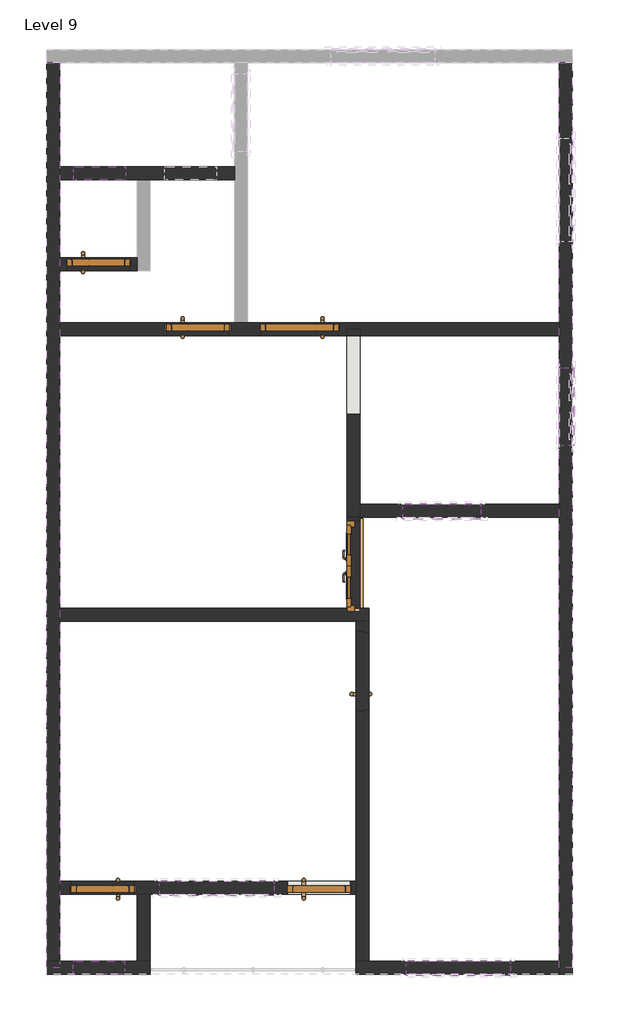
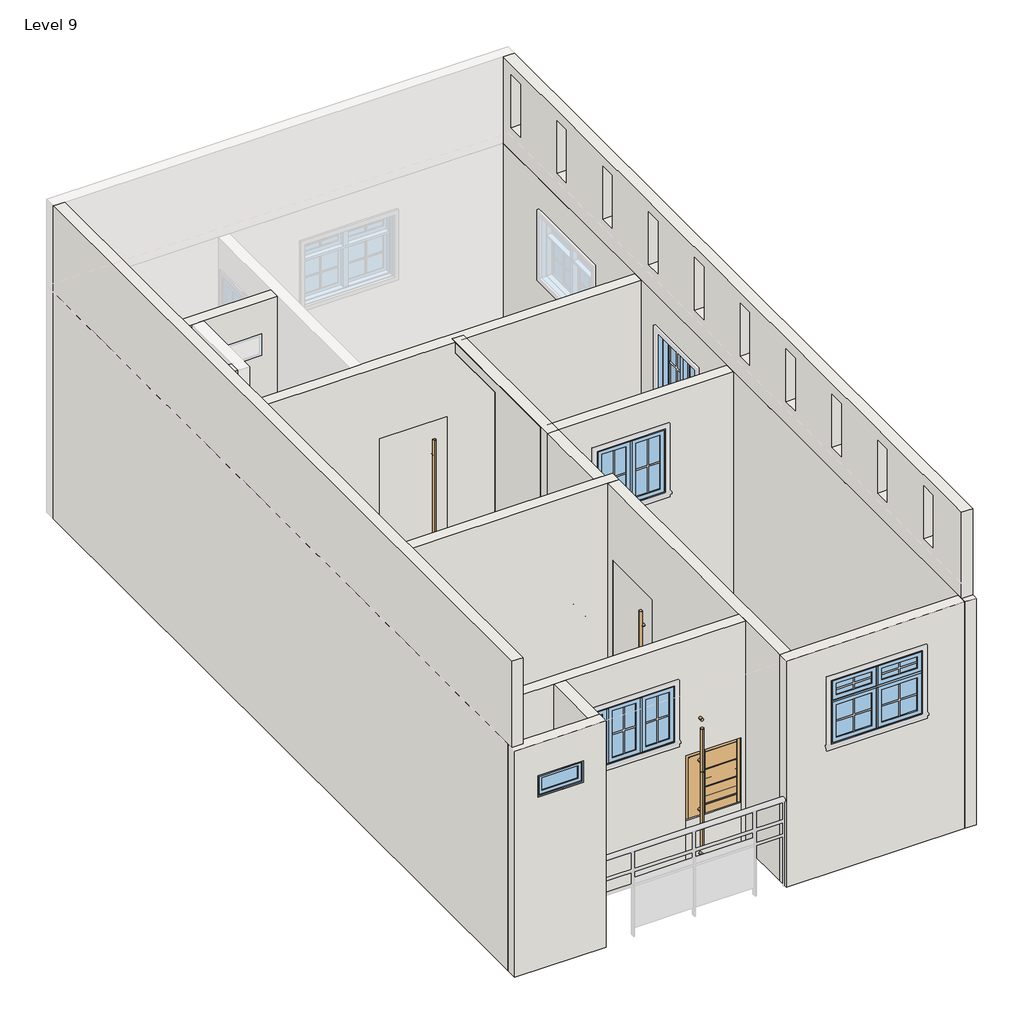
# One storey, part 1 of 2: 25 walls, 8 doors, 8 windows.
# Revit data of these elements (continued)
# Elements 6, 7 (IfcDoor, "3'") (continued)
#   Phase Created = New Construction
# Element 8 (IfcDoor, "ExtDbl (8) : 3'6\"")
#   Phase Created = New Construction
#   Materials on its faces: "Door - Panel", "Door - Handle", "Door - Glazing"
# Elements 9, 10, 11, 12 (IfcWall, "Generic - 6\"")
#   Top Offset = 0' - 0"
#   Base Offset = 0' - 0"
#   Unconnected Height = 10' - 6"
#   wall height = 10' - 6"
#   Phase Created = New Construction
#   Base Constraint = Level 9
#   Materials on its faces: "Default Wall", "Parking Stripe"
# Elements 13, 14, 15, 16, 17, 18, 19, 20, 21, 22, 23, 24, 25, 26, 27, 28, 29, 30, 31 (IfcWall, "Generic - 6\"")
#   Top Offset = 0' - 0"
#   Base Offset = 0' - 0"
#   Unconnected Height = 10' - 6"
#   wall height = 10' - 6"
#   Phase Created = New Construction
#   Base Constraint = Level 9
#   Materials on its faces: "Default Wall"
# Elements 32, 33 (IfcWall, "Generic - 6\"")
#   built-in parameter 1001111 = 10' - 6"
#   Top Offset = 0' - 0"
#   Base Offset = 10' - 6"
#   Unconnected Height = 4' - 0"
#   wall height = 4' - 0"
#   Phase Created = New Construction
#   Base Constraint = Level 9
#   Materials on its faces: "Default Wall", "WALL"
# Element 34 (IfcWindow, "Fixed : 2'")
#   Mark = "158"
#   Phase Created = New Construction
#   Materials on its faces: "Sash", "Glass"
# Element 35 (IfcWindow, "Fixed : 2'")
#   Mark = "159"
#   Phase Created = New Construction
#   Materials on its faces: "Sash", "Glass"
# Element 36 (IfcWindow, "M_Window-Awning-Triple-Horizontal : 4'5\"")
#   Mark = "157"
#   Window Inset = 0' - 0"
#   Interior Wall Closure = 0' - 2.15551"
#   Frame Extension = 0' - 0 1/4"
#   Exterior Wall Closure = 0' - 1 1/4"
#   Interior Trim Visibility = yes
#   Exterior Trim Visibility = yes
#   Phase Created = New Construction
#   Materials on its faces: "Wood - Stained", "Glass", "Clad - White"
# Element 37 (IfcWindow, "M_Window-Awning-Triple-Horizontal : 4'5\"")
#   Mark = "167"
#   Window Inset = 0' - 0"
#   Interior Wall Closure = 0' - 2.15551"
#   Frame Extension = 0' - 0 1/4"
#   Exterior Wall Closure = 0' - 1 1/4"
#   Interior Trim Visibility = yes
#   Exterior Trim Visibility = yes
#   Phase Created = New Construction
#   Materials on its faces: "Wood - Stained", "Glass", "Clad - White"
# Element 38 (IfcWindow, "M_Window-Casement-Double : 3'")
#   Mark = "154"
#   Window Inset = 0' - 0"
#   Interior Wall Closure = 0' - 2.15551"
#   Frame Extension = 0' - 0 1/4"
#   Exterior Wall Closure = 0' - 1.25197"
#   Interior Trim Visibility = yes
#   Exterior Trim Visibility = yes
#   Phase Created = New Construction
#   Materials on its faces: "Wood - Stained", "Glass", "Clad - White"
# Element 39 (IfcWindow, "M_Window-Casement-Double : 3'")
#   Mark = "155"
#   Window Inset = 0' - 0"
#   Interior Wall Closure = 0' - 2.15551"
#   Frame Extension = 0' - 0 1/4"
#   Exterior Wall Closure = 0' - 1.25197"
#   Interior Trim Visibility = yes
#   Exterior Trim Visibility = yes
#   Phase Created = New Construction
#   Materials on its faces: "Wood - Stained", "Glass", "Clad - White"
# Element 40 (IfcWindow, "M_Window-Casement-Double : 3'")
#   Mark = "164"
#   Window Inset = 0' - 0"
#   Interior Wall Closure = 0' - 2.15551"
#   Frame Extension = 0' - 0 1/4"
#   Exterior Wall Closure = 0' - 1.25197"
#   Interior Trim Visibility = yes
#   Exterior Trim Visibility = yes
#   Phase Created = New Construction
#   Materials on its faces: "Wood - Stained", "Glass", "Clad - White"
# Element 41 (IfcWindow, "M_Window-Casement-Double-Awning-Double : 4'")
#   Mark = "153"
#   Window Inset = 0' - 0"
#   Interior Wall Closure = 0' - 2.15551"
#   Frame Extension = 0' - 0 1/4"
#   Exterior Wall Closure = 0' - 1.25197"
#   Interior Trim Visibility = yes
#   Exterior Trim Visibility = yes
#   Phase Created = New Construction
#   Materials on its faces: "Wood - Stained", "Glass", "Clad - White"
# Materials
#   "Door - Glazing": colour RGB 0 0 255, transparency 0.75
#   "Door - Panel": class "Wood", colour RGB 114 82 51, transparency 0
#   "Door - Handle": colour RGB 247 247 247, transparency 0
#   "Glass": class "Glass", colour RGB 218 227 224, transparency 0.85, Description = "Soda Lime Glass", Cost = 0
#   "Sash": class "Wood", colour RGB 136 99 55, transparency 0
#   "Wood - Stained": class "Wood", colour RGB 227 170 128, transparency 0, Cost = 0
#   "Clad - White": class "Wood", colour RGB 242 242 238, transparency 0, Cost = 0
#   "Default Wall": colour RGB 80 80 80, transparency 0
#   "Parking Stripe": class "Paint", colour RGB 226 219 42, transparency 0
#   "WALL": class "Generic", colour RGB 120 120 120, transparency 0, Cost = 0
